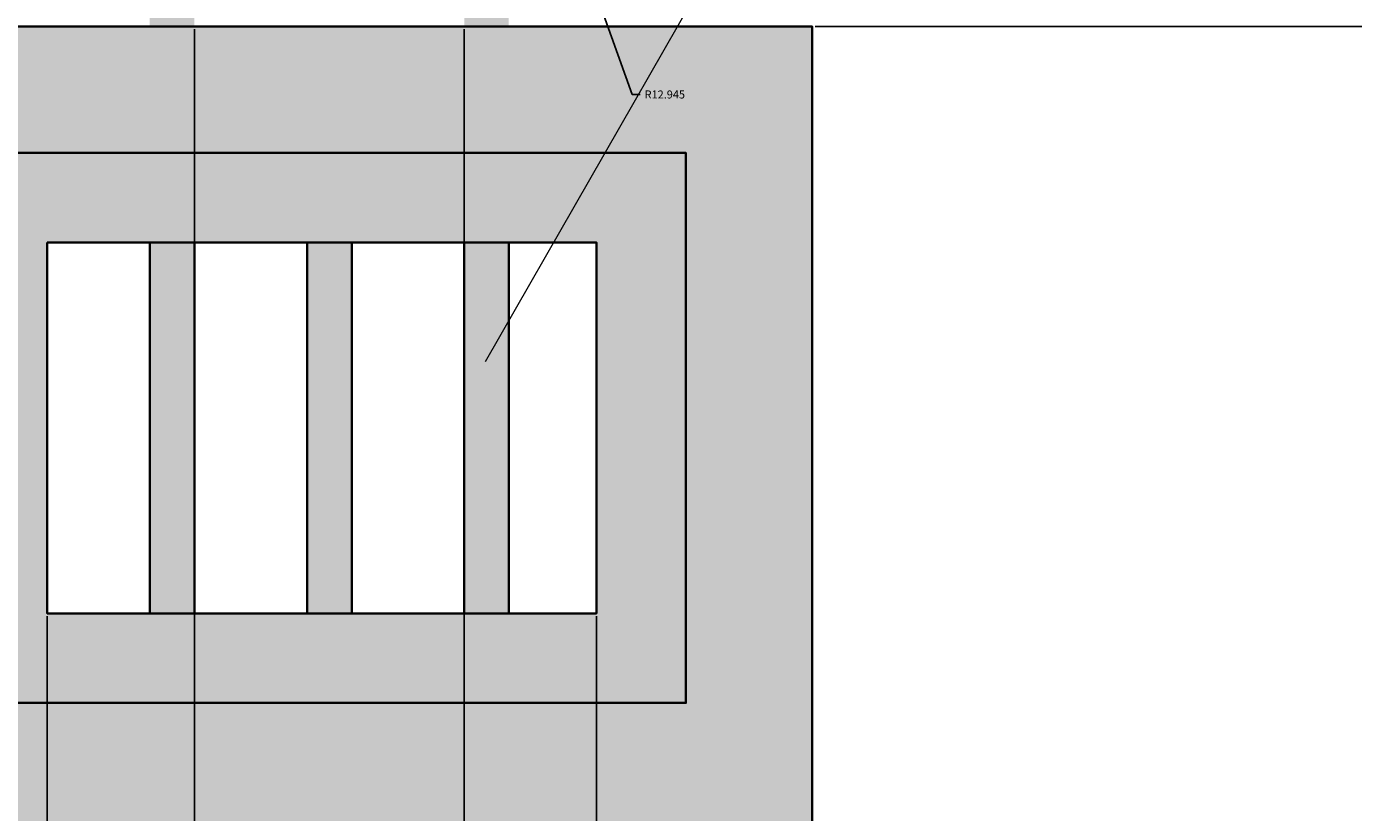
# Model space of a CAD drawing. Units: inches. Extents: x -1 to 292, y -3 to 199.
# Tile 45 of 52: x 237 to 267, y 63 to 81. Entities that reach past the tile are written whole.
import ezdxf

# ---------------------------------------------------------------- set-up
doc = ezdxf.new("R2010")
doc.units = ezdxf.units.IN
doc.header["$MEASUREMENT"] = 0
for name, color, linetype, lineweight in [('M-ANNO-LEAD', 2, 'Continuous', 18), ('M-DIMS', 2, 'Continuous', 18), ('M-EQPM', 7, 'Continuous', 35), ('M-PATT', 8, 'Continuous', 13)]:
    doc.layers.add(name, color=color, linetype=linetype, lineweight=lineweight)
doc.styles.get("Standard").update_dxf_attribs({"font": 'arial.ttf'})
doc.dimstyles.get("Standard").update_dxf_attribs({"dimtxt": 0.18, "dimasz": 0.18, "dimexe": 0.18, "dimexo": 0.0625, "dimgap": 0.09, "dimtad": 0, "dimtih": 1, "dimtoh": 1, "dimdec": 4, "dimzin": 0, "dimdsep": 46, "dimtxsty": 'Standard', "dimcen": 0.09, "dimadec": 0, "dimazin": 0, "dimtfac": 1, "dimtdec": 4, "dimtofl": 0, "dimtmove": 0, "dimatfit": 3, "dimfxl": 1, "dimtolj": 1, "dimtzin": 0, "dimarcsym": 0})

# ---------------------------------------------------------------- blocks, each defined once
blk = doc.blocks.new('*D10')
at = {"layer": 'Defpoints', "color": 0, "transparency": 16777216}
for p in [(169.176, 99.774), (169.176, 43.391), (292.04, 43.391)]:
    blk.add_point(p, dxfattribs=at)
at = {"layer": 'M-DIMS', "color": 0, "lineweight": -2, "transparency": 16777216}
for p, q in [((169.239, 99.774), (292.22, 99.774)), ((292.04, 99.594), (292.04, 71.764)), ((292.04, 43.571), (292.04, 71.4)), ((169.239, 43.391), (292.22, 43.391))]:
    blk.add_line(p, q, dxfattribs=at)
at = {"layer": 'M-DIMS', "color": 0, "transparency": 16777216}
for points in [[(292.01, 99.594), (292.07, 99.594), (292.04, 99.774)], [(292.01, 43.571), (292.07, 43.571), (292.04, 43.391)]]:
    blk.add_solid(points, dxfattribs=at)
at = {"layer": 'M-DIMS', "color": 0, "transparency": 16777216, "insert": (292.04, 71.582), "char_height": 0.18, "attachment_point": 5}
blk.add_mtext('\\A1;56.38', dxfattribs=at)
blk = doc.blocks.new('*D25')
at = {"layer": 'Defpoints', "color": 0, "transparency": 16777216}
for p in [(273.066, 88.419), (215.241, 88.13), (273.066, -2.71)]:
    blk.add_point(p, dxfattribs=at)
at = {"layer": 'M-DIMS', "color": 0, "lineweight": -2, "transparency": 16777216}
for p, q in [((273.066, 88.357), (273.066, -2.89)), ((215.241, 88.068), (215.241, -2.89)), ((215.421, -2.71), (243.76, -2.71)), ((272.886, -2.71), (244.547, -2.71))]:
    blk.add_line(p, q, dxfattribs=at)
at = {"layer": 'M-DIMS', "color": 0, "transparency": 16777216}
for points in [[(215.421, -2.68), (215.421, -2.74), (215.241, -2.71)], [(272.886, -2.68), (272.886, -2.74), (273.066, -2.71)]]:
    blk.add_solid(points, dxfattribs=at)
at = {"layer": 'M-DIMS', "color": 0, "transparency": 16777216, "insert": (244.153, -2.71), "char_height": 0.18, "attachment_point": 5}
blk.add_mtext('\\A1;57.83', dxfattribs=at)
blk = doc.blocks.new('*D28')
at = {"layer": 'Defpoints', "color": 0, "transparency": 16777216}
for p in [(241.044, 80.582), (247.095, 80.582), (247.095, -2.71)]:
    blk.add_point(p, dxfattribs=at)
at = {"layer": 'M-DIMS', "color": 0, "lineweight": -2, "transparency": 16777216}
for p, q in [((241.044, 80.52), (241.044, -2.89)), ((247.095, 80.52), (247.095, -2.89)), ((241.224, -2.71), (243.692, -2.71)), ((246.915, -2.71), (244.446, -2.71))]:
    blk.add_line(p, q, dxfattribs=at)
at = {"layer": 'M-DIMS', "color": 0, "transparency": 16777216}
for points in [[(241.224, -2.68), (241.224, -2.74), (241.044, -2.71)], [(246.915, -2.68), (246.915, -2.74), (247.095, -2.71)]]:
    blk.add_solid(points, dxfattribs=at)
at = {"layer": 'M-DIMS', "color": 0, "transparency": 16777216, "insert": (244.069, -2.71), "char_height": 0.18, "attachment_point": 5}
blk.add_mtext('\\A1;6.051', dxfattribs=at)
blk = doc.blocks.new('*D29')
at = {"layer": 'Defpoints', "color": 0, "transparency": 16777216}
for p in [(243.903, 98.567), (243.903, 44.598), (292.04, 44.598)]:
    blk.add_point(p, dxfattribs=at)
at = {"layer": 'M-DIMS', "color": 0, "lineweight": -2, "transparency": 16777216}
for p, q in [((243.966, 98.567), (292.22, 98.567)), ((292.04, 98.387), (292.04, 71.764)), ((292.04, 44.778), (292.04, 71.4)), ((243.966, 44.598), (292.22, 44.598))]:
    blk.add_line(p, q, dxfattribs=at)
at = {"layer": 'M-DIMS', "color": 0, "transparency": 16777216}
for points in [[(292.01, 98.387), (292.07, 98.387), (292.04, 98.567)], [(292.01, 44.778), (292.07, 44.778), (292.04, 44.598)]]:
    blk.add_solid(points, dxfattribs=at)
at = {"layer": 'M-DIMS', "color": 0, "transparency": 16777216, "insert": (292.04, 71.582), "char_height": 0.18, "attachment_point": 5}
blk.add_mtext('\\A1;53.97', dxfattribs=at)
blk = doc.blocks.new('*D31')
at = {"layer": 'Defpoints', "color": 0, "transparency": 16777216}
for p in [(254.903, 80.582), (292.04, 80.582), (254.903, 62.582)]:
    blk.add_point(p, dxfattribs=at)
at = {"layer": 'M-DIMS', "color": 0, "lineweight": -2, "transparency": 16777216}
for p, q in [((254.966, 80.582), (292.22, 80.582)), ((292.04, 80.402), (292.04, 71.764)), ((292.04, 62.762), (292.04, 71.4)), ((254.966, 62.582), (292.22, 62.582))]:
    blk.add_line(p, q, dxfattribs=at)
at = {"layer": 'M-DIMS', "color": 0, "transparency": 16777216}
for points in [[(292.01, 80.402), (292.07, 80.402), (292.04, 80.582)], [(292.01, 62.762), (292.07, 62.762), (292.04, 62.582)]]:
    blk.add_solid(points, dxfattribs=at)
at = {"layer": 'M-DIMS', "color": 0, "transparency": 16777216, "insert": (292.04, 71.582), "char_height": 0.18, "attachment_point": 5}
blk.add_mtext('\\A1;18', dxfattribs=at)
blk = doc.blocks.new('*D32')
at = {"layer": 'Defpoints', "color": 0, "transparency": 16777216}
for p in [(237.744, 67.423), (250.063, 67.423), (250.063, -2.71)]:
    blk.add_point(p, dxfattribs=at)
at = {"layer": 'M-DIMS', "color": 0, "lineweight": -2, "transparency": 16777216}
for p, q in [((237.744, 67.36), (237.744, -2.89)), ((250.063, 67.36), (250.063, -2.89)), ((237.924, -2.71), (243.448, -2.71)), ((249.883, -2.71), (244.359, -2.71))]:
    blk.add_line(p, q, dxfattribs=at)
at = {"layer": 'M-DIMS', "color": 0, "transparency": 16777216}
for points in [[(237.924, -2.68), (237.924, -2.74), (237.744, -2.71)], [(249.883, -2.68), (249.883, -2.74), (250.063, -2.71)]]:
    blk.add_solid(points, dxfattribs=at)
at = {"layer": 'M-DIMS', "color": 0, "transparency": 16777216, "insert": (243.903, -2.71), "char_height": 0.18, "attachment_point": 5}
blk.add_mtext('\\A1;12.319', dxfattribs=at)
blk = doc.blocks.new('*D33')
at = {"layer": 'Defpoints', "color": 0, "transparency": 16777216}
for p in [(242.955, 125.727), (292.04, 125.727), (237.933, 30.73)]:
    blk.add_point(p, dxfattribs=at)
at = {"layer": 'M-DIMS', "color": 0, "lineweight": -2, "transparency": 16777216}
for p, q in [((243.018, 125.727), (292.22, 125.727)), ((292.04, 125.547), (292.04, 78.41)), ((292.04, 30.91), (292.04, 78.046)), ((237.996, 30.73), (292.22, 30.73))]:
    blk.add_line(p, q, dxfattribs=at)
at = {"layer": 'M-DIMS', "color": 0, "transparency": 16777216}
for points in [[(292.01, 125.547), (292.07, 125.547), (292.04, 125.727)], [(292.01, 30.91), (292.07, 30.91), (292.04, 30.73)]]:
    blk.add_solid(points, dxfattribs=at)
at = {"layer": 'M-DIMS', "color": 0, "transparency": 16777216, "insert": (292.04, 78.228), "char_height": 0.18, "attachment_point": 5}
blk.add_mtext('\\A1;95', dxfattribs=at)
blk = doc.blocks.new('*D35')
at = {"layer": 'Defpoints', "color": 0, "transparency": 16777216}
for p in [(243.903, 98.567), (248.254, 86.374)]:
    blk.add_point(p, dxfattribs=at)
at = {"layer": 'M-DIMS', "color": 0, "lineweight": -2, "transparency": 16777216}
for p, q in [((243.813, 98.567), (243.993, 98.567)), ((243.903, 98.477), (243.903, 98.657)), ((250.864, 79.059), (248.314, 86.205)), ((251.044, 79.059), (250.864, 79.059))]:
    blk.add_line(p, q, dxfattribs=at)
at = {"layer": 'M-DIMS', "color": 0, "transparency": 16777216}
blk.add_solid([(248.343, 86.215), (248.286, 86.195), (248.254, 86.374)], dxfattribs=at)
at = {"layer": 'M-DIMS', "color": 0, "transparency": 16777216, "insert": (251.595, 79.059), "char_height": 0.18, "attachment_point": 5}
blk.add_mtext('\\A1;R12.945', dxfattribs=at)

msp = doc.modelspace()

# ---------------------------------------------------------------- hatches: boundary and pattern name
at = {"layer": 'M-PATT'}
h = msp.add_hatch(color=256, dxfattribs=at)
h.set_gradient(color1=(0, 255, 255), color2=(0, 255, 255), tint=1, name='CYLINDER')
h.paths.add_polyline_path([(241.0437, 75.7414), (240.0437, 75.7414), (240.0437, 67.4228), (241.0437, 67.4228)])
h.paths.add_polyline_path([(241.0437, 62.5821), (240.0437, 62.5821), (240.0437, 53.2217, -0.0283388), (241.0437, 53.6028)])
h.paths.add_polyline_path([(241.0437, 85.9411, -0.0200063), (240.0437, 86.21), (240.0437, 80.5821), (241.0437, 80.5821)])
h.paths.add_polyline_path([(248.0947, 86.3186, -0.0201581), (247.0947, 86.0208), (247.0947, 80.5821), (248.0947, 80.5821)])
h.paths.add_polyline_path([(244.5758, 75.7414), (243.5758, 75.7414), (243.5758, 67.4228), (244.5758, 67.4228)])
h.paths.add_polyline_path([(248.0947, 75.7414), (247.0947, 75.7414), (247.0947, 67.4228), (248.0947, 67.4228)])
h.paths.add_polyline_path([(248.0947, 62.5821), (247.0947, 62.5821), (247.0947, 53.4907, -0.0287763), (248.0947, 53.0654)])
h = msp.add_hatch(color=256, dxfattribs=at)
h.set_gradient(color1=(242, 103, 34), color2=(242, 103, 34), tint=1, name='CYLINDER')
h.paths.add_polyline_path([(232.9033, 62.5821), (254.9033, 62.5821), (254.9033, 80.5821), (251.8779, 80.5821), (250.2521, 77.7473), (252.0686, 77.7473), (252.0686, 65.4168), (235.7381, 65.4168), (235.7381, 77.7473), (250.2521, 77.7473), (251.8779, 80.5821), (232.9033, 80.5821)])
h = msp.add_hatch(color=256, dxfattribs=at)
h.set_gradient(color1=(76, 38, 47), color2=(76, 38, 47), tint=1, name='CYLINDER')
h.paths.add_polyline_path([(237.744, 67.4228), (237.744, 75.7414), (249.1016, 75.7414), (250.2521, 77.7473), (235.7381, 77.7473), (235.7381, 65.4168), (252.0686, 65.4168), (252.0686, 77.7473), (250.2521, 77.7473), (249.1016, 75.7414), (250.0626, 75.7414), (250.0626, 67.4228)])

# ---------------------------------------------------------------- linework, layer by layer
at = {"layer": 'M-ANNO-LEAD'}
msp.add_line((247.5701, 73.0711), (262.2218, 98.6175), dxfattribs=at)
at = {"layer": 'M-EQPM'}
for p, q in [((240.0437, 75.7414), (240.0437, 67.4228)), ((241.0437, 75.7414), (241.0437, 67.4228)), ((243.5758, 75.7414), (243.5758, 67.4228)), ((244.5758, 75.7414), (244.5758, 67.4228)), ((247.0947, 75.7414), (247.0947, 67.4228)), ((248.0947, 75.7414), (248.0947, 67.4228))]:
    msp.add_line(p, q, dxfattribs=at)
for points in [[(232.9033, 80.5821), (254.9033, 80.5821), (254.9033, 62.5821), (232.9033, 62.5821)], [(235.7381, 77.7473), (252.0686, 77.7473), (252.0686, 65.4168), (235.7381, 65.4168)], [(237.744, 75.7414), (250.0626, 75.7414), (250.0626, 67.4228), (237.744, 67.4228)]]:
    msp.add_lwpolyline(points, close=True, dxfattribs=at)

# ---------------------------------------------------------------- dimensions: what is measured, and where the dimension line sits
at = {"layer": 'M-DIMS'}
for base, p1, p2, override, picture, middle in [((292.0399, 125.7269), (237.9333, 30.7296), (242.9552, 125.7269), {"dimdec": 0, "dimlfac": 1, "dimrnd": 0, "dimzin": 0, "dimdsep": 46, "dimlunit": 2}, '*D33', (292.0399, 78.2282)), ((292.0399, 43.3906), (169.176, 99.7735), (169.176, 43.3906), {"dimdec": 2, "dimlfac": 1, "dimrnd": 0, "dimzin": 0, "dimdsep": 46, "dimlunit": 2}, '*D10', (292.0399, 71.5821)), ((292.0399, 44.5975), (243.9033, 98.5666), (243.9033, 44.5975), {"dimdec": 2, "dimlfac": 1, "dimrnd": 0, "dimzin": 0, "dimdsep": 46, "dimlunit": 2}, '*D29', (292.0399, 71.5821)), ((292.0399, 80.5821), (254.9033, 62.5821), (254.9033, 80.5821), {"dimdec": 0, "dimlfac": 1, "dimrnd": 0, "dimzin": 0, "dimdsep": 46, "dimlunit": 2}, '*D31', (292.0399, 71.5821))]:
    dim = msp.add_linear_dim(base=base, p1=p1, p2=p2, angle=90, dimstyle='Standard', override=override, dxfattribs=at)
    dim.commit()
    dim.dimension.update_dxf_attribs({"geometry": picture, "text_midpoint": middle})
dim = msp.add_radius_dim(center=(243.9033, 98.5666), mpoint=(248.2539, 86.3742), dimstyle='Standard', override={"dimdec": 3, "dimlfac": 1, "dimrnd": 0, "dimzin": 0, "dimdsep": 46, "dimlunit": 2}, dxfattribs=at)
dim.commit()
dim.dimension.update_dxf_attribs({"geometry": '*D35', "text_midpoint": (251.5947, 79.0588), "dimtype": 164})
for base, p1, p2, override, picture, middle in [((273.0659, -2.7104), (215.2407, 88.1304), (273.0659, 88.4191), {"dimdec": 2, "dimlfac": 1, "dimrnd": 0, "dimzin": 0, "dimdsep": 46, "dimlunit": 2}, '*D25', (244.1533, -2.7104)), ((247.0947, -2.7104), (241.0437, 80.5821), (247.0947, 80.5821), {"dimdec": 3, "dimlfac": 1, "dimrnd": 0, "dimzin": 0, "dimdsep": 46, "dimlunit": 2}, '*D28', (244.0692, -2.7104)), ((250.0626, -2.7104), (237.744, 67.4228), (250.0626, 67.4228), {"dimdec": 3, "dimlfac": 1, "dimrnd": 0, "dimzin": 0, "dimdsep": 46, "dimlunit": 2}, '*D32', (243.9033, -2.7104))]:
    dim = msp.add_linear_dim(base=base, p1=p1, p2=p2, dimstyle='Standard', override=override, dxfattribs=at)
    dim.commit()
    dim.dimension.update_dxf_attribs({"geometry": picture, "text_midpoint": middle})

doc.saveas('drawing.dxf')
